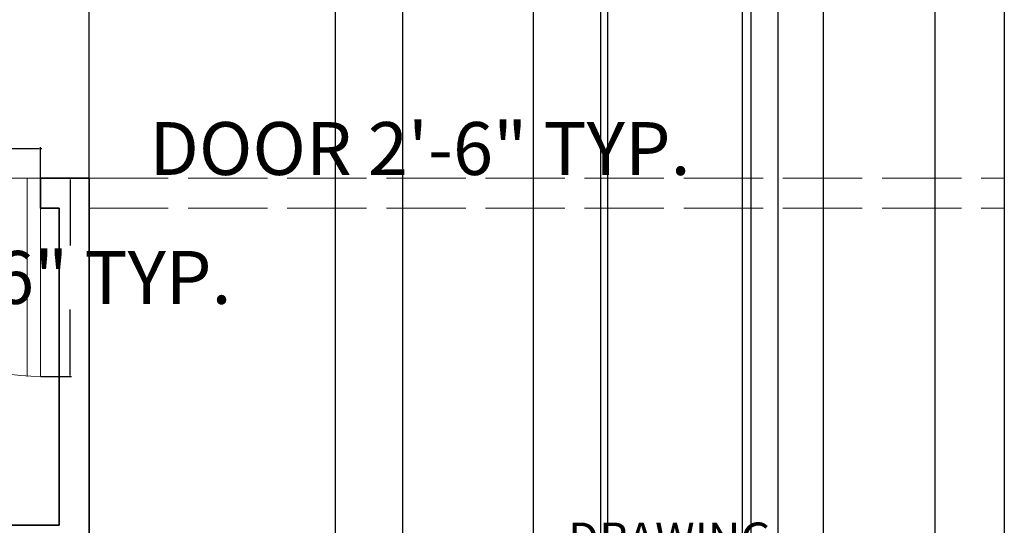
# Model space of a CAD drawing. Units: inches. Extents: x -26 to 385, y 12 to 697.
# Tile 10 of 13: x 136 to 285, y 280 to 356. Entities that reach past the tile are written whole.
import ezdxf

# ---------------------------------------------------------------- set-up
doc = ezdxf.new("R2010")
doc.units = ezdxf.units.IN
doc.header["$MEASUREMENT"] = 0
doc.linetypes.add('ACAD_ISO02W100', pattern=[15, 12, -3])
for name, color, linetype, lineweight in [('A-ANNO-DIMS', 4, 'Continuous', 18), ('A-AREA-IDEN', 4, 'Continuous', 18), ('A-DOOR', 30, 'Continuous', 20), ('A-FLOR-OVHD', 3, 'ACAD_ISO02W100', 13), ('A-WALL', 40, 'Continuous', 35)]:
    doc.layers.add(name, color=color, linetype=linetype, lineweight=lineweight)
doc.styles.get("Standard").update_dxf_attribs({"font": 'italic8.shx'})
doc.dimstyles.get("Standard").update_dxf_attribs({"dimtxt": 8, "dimasz": 0.18, "dimexe": 0.18, "dimexo": 0.0625, "dimgap": 0.09, "dimtad": 0, "dimtih": 1, "dimtoh": 1, "dimdec": 4, "dimzin": 0, "dimdsep": 46, "dimlunit": 3, "dimtxsty": 'Standard', "dimcen": 0.09, "dimclrd": 2, "dimclre": 3, "dimclrt": 6, "dimadec": 0, "dimazin": 0, "dimtfac": 1, "dimtdec": 4, "dimtofl": 0, "dimtmove": 0, "dimatfit": 3, "dimfxl": 1, "dimtolj": 1, "dimtzin": 0, "dimarcsym": 0})

# ---------------------------------------------------------------- blocks, each defined once
blk = doc.blocks.new('DOOR-SWING-30IN')
for p, q in [((0, -30), (0, 0)), ((0, 0), (30, 0)), ((0, -2), (30, -2))]:
    blk.add_line(p, q)
blk.add_arc((0, 0), 30, 270, 0)
blk = doc.blocks.new('*D17')
at = {"layer": 'A-ANNO-DIMS', "color": 3, "lineweight": -2, "transparency": 16777216}
for p, q in [((108.79, 332.44), (108.79, 337.06)), ((138.79, 332.44), (138.79, 337.06))]:
    blk.add_line(p, q, dxfattribs=at)
at = {"layer": 'A-ANNO-DIMS', "color": 2, "lineweight": -2, "transparency": 16777216}
for p, q in [((108.97, 336.88), (138.61, 336.88)), ((138.79, 336.88), (138.97, 336.88))]:
    blk.add_line(p, q, dxfattribs=at)
at = {"layer": 'A-ANNO-DIMS', "color": 2, "transparency": 16777216}
for points in [[(108.97, 336.91), (108.97, 336.85), (108.79, 336.88)], [(138.61, 336.91), (138.61, 336.85), (138.79, 336.88)]]:
    blk.add_solid(points, dxfattribs=at)
at = {"layer": 'Defpoints', "color": 0, "transparency": 16777216}
for p in [(138.79, 336.88), (108.79, 332.38), (138.79, 332.38)]:
    blk.add_point(p, dxfattribs=at)
at = {"layer": 'A-ANNO-DIMS', "color": 6, "transparency": 16777216, "insert": (196.21, 336.88), "char_height": 8, "attachment_point": 5}
blk.add_mtext('\\A1;DOOR 2\'-6" TYP.', dxfattribs=at)
blk = doc.blocks.new('*D18')
at = {"layer": 'A-ANNO-DIMS', "color": 3, "lineweight": -2, "transparency": 16777216}
for p, q in [((138.86, 332.38), (143.47, 332.38)), ((138.86, 302.38), (143.47, 302.38))]:
    blk.add_line(p, q, dxfattribs=at)
at = {"layer": 'A-ANNO-DIMS', "color": 2, "lineweight": -2, "transparency": 16777216}
for p, q in [((143.29, 332.2), (143.29, 322.23)), ((143.29, 302.56), (143.29, 312.53))]:
    blk.add_line(p, q, dxfattribs=at)
at = {"layer": 'A-ANNO-DIMS', "color": 2, "transparency": 16777216}
for points in [[(143.26, 332.2), (143.32, 332.2), (143.29, 332.38)], [(143.26, 302.56), (143.32, 302.56), (143.29, 302.38)]]:
    blk.add_solid(points, dxfattribs=at)
at = {"layer": 'Defpoints', "color": 0, "transparency": 16777216}
for p in [(138.79, 332.38), (138.79, 302.38), (143.29, 302.38)]:
    blk.add_point(p, dxfattribs=at)
at = {"layer": 'A-ANNO-DIMS', "color": 6, "transparency": 16777216, "insert": (143.29, 317.38), "char_height": 8, "attachment_point": 5}
blk.add_mtext('\\A1;2\'-6" TYP.', dxfattribs=at)
blk = doc.blocks.new('*D25')
at = {"layer": 'A-ANNO-DIMS', "color": 3, "lineweight": -2, "transparency": 16777216}
for p, q in [((284.629322, 368.316588), (284.629322, 23.949088)), ((320.629322, 368.316588), (320.629322, 23.949088))]:
    blk.add_line(p, q, dxfattribs=at)
at = {"layer": 'A-ANNO-DIMS', "color": 2, "lineweight": -2, "transparency": 16777216}
for p, q in [((284.449322, 24.129088), (284.269322, 24.129088)), ((320.809322, 24.129088), (320.989322, 24.129088))]:
    blk.add_line(p, q, dxfattribs=at)
at = {"layer": 'A-ANNO-DIMS', "color": 2, "transparency": 16777216}
for points in [[(284.449322, 24.159088), (284.449322, 24.099088), (284.629322, 24.129088)], [(320.809322, 24.159088), (320.809322, 24.099088), (320.629322, 24.129088)]]:
    blk.add_solid(points, dxfattribs=at)
at = {"layer": 'Defpoints', "color": 0, "transparency": 16777216}
for p in [(284.629322, 368.379088), (320.629322, 368.379088), (320.629322, 24.129088)]:
    blk.add_point(p, dxfattribs=at)
at = {"layer": 'A-ANNO-DIMS', "color": 6, "transparency": 16777216, "insert": (302.629322, 24.129088), "char_height": 8, "attachment_point": 5}
blk.add_mtext('\\A1;3\'-0"', dxfattribs=at)
blk = doc.blocks.new('*D35')
at = {"layer": 'A-ANNO-DIMS', "color": 3, "lineweight": -2, "transparency": 16777216}
for p, q in [((193.6, 147.94), (193.6, 684.81)), ((244.99, 147.94), (244.99, 684.81))]:
    blk.add_line(p, q, dxfattribs=at)
at = {"layer": 'A-ANNO-DIMS', "color": 2, "lineweight": -2, "transparency": 16777216}
for p, q in [((193.78, 684.63), (244.81, 684.63)), ((244.99, 684.63), (245.17, 684.63))]:
    blk.add_line(p, q, dxfattribs=at)
at = {"layer": 'A-ANNO-DIMS', "color": 2, "transparency": 16777216}
for points in [[(193.78, 684.66), (193.78, 684.6), (193.6, 684.63)], [(244.81, 684.66), (244.81, 684.6), (244.99, 684.63)]]:
    blk.add_solid(points, dxfattribs=at)
at = {"layer": 'Defpoints', "color": 0, "transparency": 16777216}
for p in [(244.99, 684.63), (193.6, 147.88), (244.99, 147.88)]:
    blk.add_point(p, dxfattribs=at)
at = {"layer": 'A-ANNO-DIMS', "color": 6, "transparency": 16777216, "insert": (278.4, 684.63), "char_height": 8, "attachment_point": 5}
blk.add_mtext('\\A1;4\'-3 1/2"', dxfattribs=at)
blk = doc.blocks.new('*D36')
at = {"layer": 'A-ANNO-DIMS', "color": 3, "lineweight": -2, "transparency": 16777216}
for p, q in [((146.13, 147.94), (146.13, 684.81)), ((193.6, 147.94), (193.6, 684.81))]:
    blk.add_line(p, q, dxfattribs=at)
at = {"layer": 'A-ANNO-DIMS', "color": 2, "lineweight": -2, "transparency": 16777216}
for p, q in [((146.31, 684.63), (193.42, 684.63)), ((193.6, 684.63), (193.78, 684.63))]:
    blk.add_line(p, q, dxfattribs=at)
at = {"layer": 'A-ANNO-DIMS', "color": 2, "transparency": 16777216}
for points in [[(146.31, 684.66), (146.31, 684.6), (146.13, 684.63)], [(193.42, 684.66), (193.42, 684.6), (193.6, 684.63)]]:
    blk.add_solid(points, dxfattribs=at)
at = {"layer": 'Defpoints', "color": 0, "transparency": 16777216}
for p in [(193.6, 684.63), (146.13, 147.88), (193.6, 147.88)]:
    blk.add_point(p, dxfattribs=at)
at = {"layer": 'A-ANNO-DIMS', "color": 6, "transparency": 16777216, "insert": (228.34, 684.63), "char_height": 8, "attachment_point": 5}
blk.add_mtext('\\A1;3\'-11 1/2"', dxfattribs=at)
blk = doc.blocks.new('*D37')
at = {"layer": 'A-ANNO-DIMS', "color": 3, "lineweight": -2, "transparency": 16777216}
for p, q in [((223.55, 597.32), (223.55, 23.95)), ((257.22, 597.32), (257.22, 23.95))]:
    blk.add_line(p, q, dxfattribs=at)
at = {"layer": 'A-ANNO-DIMS', "color": 2, "lineweight": -2, "transparency": 16777216}
for p, q in [((223.73, 24.13), (257.04, 24.13)), ((257.22, 24.13), (257.4, 24.13))]:
    blk.add_line(p, q, dxfattribs=at)
at = {"layer": 'A-ANNO-DIMS', "color": 2, "transparency": 16777216}
for points in [[(223.73, 24.16), (223.73, 24.1), (223.55, 24.13)], [(257.04, 24.16), (257.04, 24.1), (257.22, 24.13)]]:
    blk.add_solid(points, dxfattribs=at)
at = {"layer": 'Defpoints', "color": 0, "transparency": 16777216}
for p in [(223.55, 597.38), (257.22, 597.38), (257.22, 24.13)]:
    blk.add_point(p, dxfattribs=at)
at = {"layer": 'A-ANNO-DIMS', "color": 6, "transparency": 16777216, "insert": (290.63, 24.13), "char_height": 8, "attachment_point": 5}
blk.add_mtext('\\A1;2\'-9 1/2"', dxfattribs=at)
blk = doc.blocks.new('*D39')
at = {"layer": 'A-ANNO-DIMS', "color": 3, "lineweight": -2, "transparency": 16777216}
for p, q in [((183.36, 597.32), (183.36, 23.95)), ((213.36, 597.32), (213.36, 23.95))]:
    blk.add_line(p, q, dxfattribs=at)
at = {"layer": 'A-ANNO-DIMS', "color": 2, "lineweight": -2, "transparency": 16777216}
for p, q in [((183.54, 24.13), (213.18, 24.13)), ((213.36, 24.13), (213.54, 24.13))]:
    blk.add_line(p, q, dxfattribs=at)
at = {"layer": 'A-ANNO-DIMS', "color": 2, "transparency": 16777216}
for points in [[(183.54, 24.16), (183.54, 24.1), (183.36, 24.13)], [(213.18, 24.16), (213.18, 24.1), (213.36, 24.13)]]:
    blk.add_solid(points, dxfattribs=at)
at = {"layer": 'Defpoints', "color": 0, "transparency": 16777216}
for p in [(183.36, 597.38), (213.36, 597.38), (213.36, 24.13)]:
    blk.add_point(p, dxfattribs=at)
at = {"layer": 'A-ANNO-DIMS', "color": 6, "transparency": 16777216, "insert": (231.53, 24.13), "char_height": 8, "attachment_point": 5}
blk.add_mtext('\\A1;2\'-6"', dxfattribs=at)
blk = doc.blocks.new('*D42')
at = {"layer": 'A-ANNO-DIMS', "color": 3, "lineweight": -2, "transparency": 16777216}
for p, q in [((250.37, 518.99), (250.37, 23.95)), ((274.13, 518.99), (274.13, 23.95))]:
    blk.add_line(p, q, dxfattribs=at)
at = {"layer": 'A-ANNO-DIMS', "color": 2, "lineweight": -2, "transparency": 16777216}
for p, q in [((250.55, 24.13), (273.95, 24.13)), ((274.13, 24.13), (274.31, 24.13))]:
    blk.add_line(p, q, dxfattribs=at)
at = {"layer": 'A-ANNO-DIMS', "color": 2, "transparency": 16777216}
for points in [[(250.55, 24.16), (250.55, 24.1), (250.37, 24.13)], [(273.95, 24.16), (273.95, 24.1), (274.13, 24.13)]]:
    blk.add_solid(points, dxfattribs=at)
at = {"layer": 'Defpoints', "color": 0, "transparency": 16777216}
for p in [(250.37, 519.05), (274.13, 519.05), (274.13, 24.13)]:
    blk.add_point(p, dxfattribs=at)
at = {"layer": 'A-ANNO-DIMS', "color": 6, "transparency": 16777216, "insert": (292.3, 24.13), "char_height": 8, "attachment_point": 5}
blk.add_mtext('\\A1;2\'-0"', dxfattribs=at)
blk = doc.blocks.new('*D46')
at = {"layer": 'A-ANNO-DIMS', "color": 3, "lineweight": -2, "transparency": 16777216}
for p, q in [((224.59, 477.32), (224.59, 23.95)), ((284.63, 477.32), (284.63, 23.95))]:
    blk.add_line(p, q, dxfattribs=at)
at = {"layer": 'A-ANNO-DIMS', "color": 2, "lineweight": -2, "transparency": 16777216}
for p, q in [((224.77, 24.13), (236.62, 24.13)), ((284.45, 24.13), (272.61, 24.13))]:
    blk.add_line(p, q, dxfattribs=at)
at = {"layer": 'A-ANNO-DIMS', "color": 2, "transparency": 16777216}
for points in [[(224.77, 24.16), (224.77, 24.1), (224.59, 24.13)], [(284.45, 24.16), (284.45, 24.1), (284.63, 24.13)]]:
    blk.add_solid(points, dxfattribs=at)
at = {"layer": 'Defpoints', "color": 0, "transparency": 16777216}
for p in [(224.59, 477.38), (284.63, 477.38), (284.63, 24.13)]:
    blk.add_point(p, dxfattribs=at)
at = {"layer": 'A-ANNO-DIMS', "color": 6, "transparency": 16777216, "insert": (254.61, 24.13), "char_height": 8, "attachment_point": 5}
blk.add_mtext('\\A1;5\'-0"', dxfattribs=at)
blk = doc.blocks.new('*D50')
at = {"layer": 'A-ANNO-DIMS', "color": 3, "lineweight": -2, "transparency": 16777216}
for p, q in [((246.28, 401.87), (246.28, 23.95)), ((284.63, 398.32), (284.63, 23.95))]:
    blk.add_line(p, q, dxfattribs=at)
at = {"layer": 'A-ANNO-DIMS', "color": 2, "lineweight": -2, "transparency": 16777216}
for p, q in [((246.46, 24.13), (284.45, 24.13)), ((284.63, 24.13), (284.81, 24.13))]:
    blk.add_line(p, q, dxfattribs=at)
at = {"layer": 'A-ANNO-DIMS', "color": 2, "transparency": 16777216}
for points in [[(246.46, 24.16), (246.46, 24.1), (246.28, 24.13)], [(284.45, 24.16), (284.45, 24.1), (284.63, 24.13)]]:
    blk.add_solid(points, dxfattribs=at)
at = {"layer": 'Defpoints', "color": 0, "transparency": 16777216}
for p in [(246.28, 401.93), (284.63, 398.38), (284.63, 24.13)]:
    blk.add_point(p, dxfattribs=at)
at = {"layer": 'A-ANNO-DIMS', "color": 6, "transparency": 16777216, "insert": (318.04, 24.13), "char_height": 8, "attachment_point": 5}
blk.add_mtext('\\A1;3\'-2 1/2"', dxfattribs=at)

msp = doc.modelspace()

# ---------------------------------------------------------------- linework, layer by layer
at = {"layer": 'A-FLOR-OVHD'}
for p, q in [((146.12932, 332.37909), (284.62932, 332.37909)), ((146.12932, 327.87909), (284.62932, 327.87909))]:
    msp.add_line(p, q, dxfattribs=at)
at = {"layer": 'A-WALL'}
for p, q in [((146.12932, 332.37909), (138.79289, 332.37909)), ((138.79289, 332.37909), (138.79289, 327.87909)), ((146.12932, 332.37909), (146.12932, 194.90341)), ((141.62932, 327.87909), (138.79289, 327.87909)), ((141.62932, 327.87909), (141.62932, 279.87909)), ((141.62932, 279.87909), (29.62932, 279.87909))]:
    msp.add_line(p, q, dxfattribs=at)

# ---------------------------------------------------------------- block references
at = {"layer": 'A-DOOR', "rotation": 269.9999999999999}
msp.add_blockref('DOOR-SWING-30IN', (138.79289, 332.37909), dxfattribs=at)

# ---------------------------------------------------------------- texts
at = {"layer": 'A-AREA-IDEN'}
msp.add_text('DRAWING', height=5, dxfattribs=at).set_placement((218.60931, 275.29915))

# ---------------------------------------------------------------- dimensions: what is measured, and where the dimension line sits
at = {"layer": 'A-ANNO-DIMS'}
for base, p1, p2, picture, middle in [((193.59818, 684.62909), (146.12932, 147.87909), (193.59818, 147.87909), '*D36', (228.34437, 684.62909)), ((244.98557, 684.62909), (193.59818, 147.87909), (244.98557, 147.87909), '*D35', (278.39843, 684.62909)), ((213.35855, 24.12909), (183.35855, 597.37909), (213.35855, 597.37909), '*D39', (231.53331, 24.12909)), ((257.21981, 24.12909), (223.54856, 597.37909), (257.21981, 597.37909), '*D37', (290.63267, 24.12909)), ((274.12932, 24.12909), (250.37102, 519.05498), (274.12932, 519.05498), '*D42', (292.30408, 24.12909)), ((284.62932, 24.12909), (224.59493, 477.37909), (284.62932, 477.37909), '*D46', (254.61213, 24.12909)), ((284.62932, 24.12909), (246.27828, 401.934), (284.62932, 398.37909), '*D50', (318.04218, 24.12909)), ((320.62932, 24.12909), (284.62932, 368.37909), (320.62932, 368.37909), '*D25', (302.62932, 24.12909))]:
    dim = msp.add_linear_dim(base=base, p1=p1, p2=p2, dimstyle='Standard', override={"dimdec": 1, "dimlfac": 1, "dimrnd": 0, "dimzin": 1, "dimdsep": 46, "dimlunit": 4, "dimfrac": 2}, dxfattribs=at)
    dim.commit()
    dim.dimension.update_dxf_attribs({"geometry": picture, "text_midpoint": middle})
dim = msp.add_linear_dim(base=(138.79289, 336.87909), p1=(108.79289, 332.37909), p2=(138.79289, 332.37909), text='DOOR <> TYP.', dimstyle='Standard', override={"dimdec": 1, "dimlfac": 1, "dimrnd": 0, "dimzin": 1, "dimdsep": 46, "dimlunit": 4, "dimfrac": 2}, dxfattribs=at)
dim.commit()
dim.dimension.update_dxf_attribs({"geometry": '*D17', "text_midpoint": (196.20575, 336.87909)})
dim = msp.add_linear_dim(base=(143.29289, 302.37909), p1=(138.79289, 332.37909), p2=(138.79289, 302.37909), angle=270, text='<> TYP.', dimstyle='Standard', override={"dimdec": 1, "dimlfac": 1, "dimrnd": 0, "dimzin": 1, "dimdsep": 46, "dimlunit": 4, "dimfrac": 2}, dxfattribs=at)
dim.commit()
dim.dimension.update_dxf_attribs({"geometry": '*D18', "text_midpoint": (143.29289, 317.37909)})

doc.saveas('drawing.dxf')
